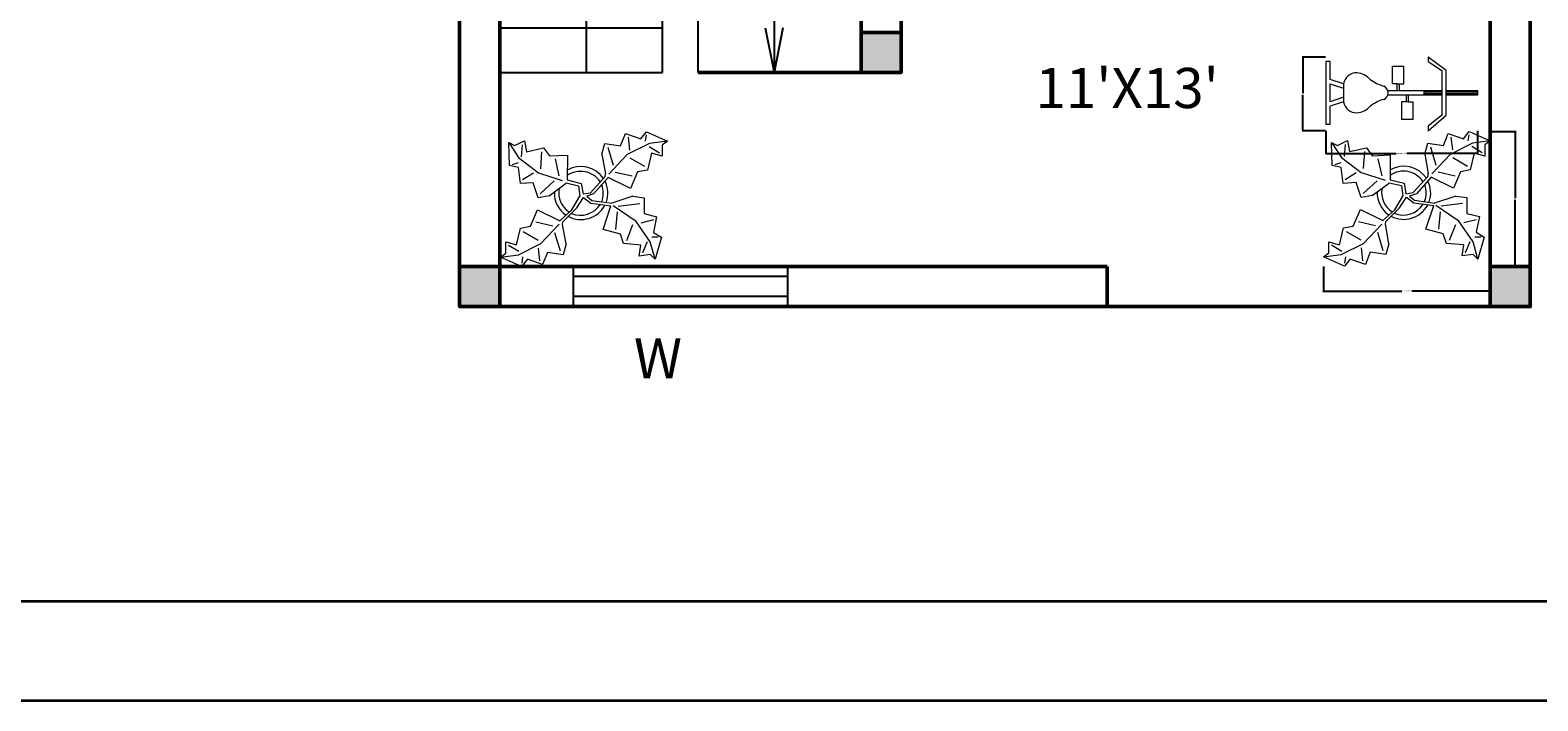
# Model space of a CAD drawing. Units: inches. Extents: x 28637 to 29820, y 17246 to 17928.
# Tile 3 of 6: x 28996 to 29334, y 17246 to 17397. Entities that reach past the tile are written whole.
import ezdxf

# ---------------------------------------------------------------- set-up
doc = ezdxf.new("R2010")
doc.units = ezdxf.units.IN
for name, color, linetype, lineweight in [('A-ANNO-DIMS', 2, 'Continuous', 18), ('A-ANNO-TEXT', 7, 'Continuous', 25), ('A-ANNO-TTLB', 7, 'Continuous', 35), ('A-AREA-IDEN', 30, 'Continuous', 25), ('A-COLS', 1, 'Continuous', 50), ('A-FLOR-STRS', 3, 'Continuous', 25), ('A-FURN', 8, 'Continuous', 18), ('A-GLAZ', 4, 'Continuous', 25), ('A-WALL', 7, 'Continuous', 50)]:
    doc.layers.add(name, color=color, linetype=linetype, lineweight=lineweight)
doc.styles.get("Standard").update_dxf_attribs({"font": 'arial.ttf'})
doc.dimstyles.get("Standard").update_dxf_attribs({"dimtxt": 0.18, "dimasz": 0.18, "dimexe": 0.18, "dimexo": 0.0625, "dimgap": 0.09, "dimtad": 0, "dimtih": 1, "dimtoh": 1, "dimdec": 4, "dimzin": 0, "dimdsep": 46, "dimtxsty": 'Standard', "dimcen": 0.09, "dimadec": 0, "dimazin": 0, "dimtfac": 1, "dimtdec": 4, "dimtofl": 0, "dimtmove": 0, "dimatfit": 3, "dimfxl": 1, "dimtolj": 1, "dimtzin": 0, "dimarcsym": 0})

# ---------------------------------------------------------------- blocks, each defined once
blk = doc.blocks.new('Exercise Bike')
for p, q in [((-0.75, 10), (-0.75, 17)), ((-0.75, 17), (0.25, 17)), ((-0.5, 17), (-0.5, 9.9929)), ((-0.25, 10), (-0.25, 17)), ((0, 17), (0, 9.9929)), ((0.25, 17), (0.25, 10)), ((-5.25, 10), (-8.25, 6)), ((-7.25, 6), (-5.25, 9)), ((-0.75, 10), (-5.25, 10)), ((-5.25, 9), (4.75, 9)), ((4.75, 10), (-0.75, 10)), ((-0.75, 5), (-0.75, 9)), ((-0.5, 8.9396), (-0.5, 5)), ((-0.25, 5), (-0.25, 9)), ((0, 8.9396), (0, 5)), ((0.25, 9), (0.25, 5)), ((8.25, 6), (4.75, 10)), ((4.75, 9), (7.25, 6)), ((-8.25, 6), (-7.25, 6)), ((-0.75, -3.0635), (-0.75, 5)), ((-0.75, 5), (0.25, 5)), ((0.25, 5), (0.25, -3.0635)), ((7.25, 6), (8.25, 6)), ((-6.25, -2), (-6.25, 0.5)), ((-2.25, 0.5), (-6.25, 0.5)), ((-2.25, -0.5), (-2.25, 0.5)), ((0.25, 1.5), (1.75, 1.5)), ((0.25, 1), (1.75, 1)), ((1.75, 2.5), (5.75, 2.5)), ((1.75, 1.5), (1.75, 2.5)), ((1.75, 1.5), (1.75, 0)), ((1.75, 0), (5.75, 0)), ((5.75, 2.5), (5.75, 0)), ((-2.25, -2), (-6.25, -2)), ((-2.25, -0.5), (-0.75, -0.5)), ((-2.25, -1), (-2.25, -0.5)), ((-2.25, -1), (-2.25, -2)), ((-0.75, -1), (-2.25, -1)), ((-2.25, -13), (-3.25, -16)), ((-2.25, -16), (-1.25, -13)), ((-2.25, -13), (1.75, -13)), ((0.75, -13), (1.75, -16)), ((1.75, -13), (2.75, -16)), ((-7.25, -16), (-7.25, -17)), ((-4.75, -16), (-7.25, -16)), ((-3.25, -16), (-4.75, -16)), ((1.75, -16), (-2.25, -16)), ((6.75, -16), (2.75, -16)), ((6.75, -17), (6.75, -16)), ((-7.25, -17), (6.75, -17))]:
    blk.add_line(p, q)
for centre, radius, start, end in [((-0.25, -4.625), 1.625, 22.61987, 157.3801), ((-9.6692, -1.9154), 8.1889, 321.6175, 345.2525), ((9.1691, -1.9154), 8.1889, 194.7476, 218.3825), ((0.1685, -10.5843), 4.9531, 133.6443, 173.2256), ((-1.7006, -10.0005), 3.0494, 179.9906, 259.6205), ((1.2006, -10.0005), 3.0494, 280.3795, 0.009389), ((-0.6686, -10.5843), 4.9531, 6.774486, 46.35562)]:
    blk.add_arc(centre, radius, start, end)
blk = doc.blocks.new('Plant - Rubber or Philodendron')
for p, q in [((13.3837, 12.301), (14.68, 13.9039)), ((14.68, 13.9039), (19.3848, 11.8146)), ((-16.2005, 11.4774), (-13.9899, 8.1064)), ((-16.2005, 11.4774), (-14.8639, 10.7964)), ((-16.0159, 6.3329), (-16.2005, 11.4774)), ((-14.8639, 10.7964), (-12.6195, 11.8975)), ((-13.3174, 8.325), (-13.0735, 11.0065)), ((-12.6195, 11.8975), (-12.1909, 9.4345)), ((-12.1909, 9.4345), (-8.3829, 10.3)), ((-8.3829, 10.3), (-7.0549, 8.501)), ((4.6914, 8.8812), (5.3859, 11.2828)), ((5.3859, 11.2828), (8.8871, 10.7908)), ((5.9878, 10.4842), (7.1971, 6.3869)), ((8.8871, 10.7908), (9.9809, 13.4933)), ((9.9809, 13.4933), (13.3837, 12.301)), ((15.3859, 11.3055), (10.3916, 8.7942)), ((10.5828, 12.6946), (10.8893, 9.7953)), ((14.5816, 13.2037), (14.3848, 11.8033)), ((15.2875, 10.6053), (17.5907, 9.2105)), ((19.3848, 11.8146), (15.3859, 11.3055)), ((19.3848, 11.8146), (18.1868, 10.9119)), ((18.1868, 10.9119), (18.1925, 8.4119)), ((-15.3434, 6.5514), (-13.9984, 6.9884)), ((-13.9899, 8.1064), (-9.5434, 4.7185)), ((-8.8369, 9.409), (-9.0894, 5.6095)), ((-7.0549, 8.501), (-3.0284, 8.6941)), ((-4.8529, 4.012), (-5.7184, 7.82)), ((-3.0284, 8.6941), (-3.0709, 3.1041)), ((4.6914, 8.8812), (5.5014, 4.4831)), ((10.3916, 8.7942), (6.2847, 4.4028)), ((14.2977, 6.1031), (10.9934, 7.9956)), ((15.7909, 9.1065), (14.8995, 5.3044)), ((18.1925, 8.4119), (15.7909, 9.1065)), ((-14.0069, 5.8704), (-16.0159, 6.3329)), ((-13.5868, 2.2894), (-14.0069, 5.8704)), ((-13.1329, 3.1804), (-10.6614, 4.727)), ((-9.5434, 4.7185), (-4.1917, 2.9888)), ((2.1141, 0.2298), (5.4346, 3.9146)), ((6.1032, 3.6844), (2.8262, -0.031)), ((5.4346, 3.9146), (5.5014, 4.4831)), ((11.1089, 1.1958), (6.1032, 3.6844)), ((7.7005, 4.8881), (11.5025, 3.9967)), ((12.7005, 4.8994), (11.1089, 1.1958)), ((14.8995, 5.3044), (12.7005, 4.8994)), ((-10.6784, 2.491), (-13.5868, 2.2894)), ((-9.5858, -0.8715), (-10.6784, 2.491)), ((-9.1318, 0.0195), (-5.9793, 2.9025)), ((-7.1228, -0.443), (-3.5248, 2.2131)), ((-3.5248, 2.2131), (-3.3011, 2.4355)), ((-3.3011, 2.4355), (-0.5306, 1.7947)), ((-3.0709, 3.1041), (0.0797, 2.3163)), ((-0.5306, 1.7947), (-0.2255, -0.5527)), ((-0.5306, 1.7947), (-0.5306, 1.7947)), ((0.0797, 2.3163), (0.4866, -0.031)), ((0.4866, -0.031), (2.1141, 0.2298)), ((-7.1228, -0.443), (-9.5858, -0.8715)), ((-4.0579, -6.2781), (-0.9375, -3.1608)), ((-2.019, -3.6148), (-0.2255, -0.5527)), ((-0.9375, -3.1608), (0.5883, -0.8135)), ((0.5883, -0.8135), (2.2447, -2.0916)), ((2.8262, -0.031), (1.3003, -0.5527)), ((1.3003, -0.5527), (2.4193, -1.4655)), ((2.2447, -2.0916), (6.7108, -2.6626)), ((2.4193, -1.4655), (6.895, -2.1175)), ((4.943, -7.9659), (6.7108, -2.6626)), ((11.6605, -0.5413), (6.895, -2.1175)), ((12.3677, -6.1981), (7.219, -2.6772)), ((8.3544, -2.7453), (13.1973, -2.1704)), ((11.6605, -0.5413), (14.1354, -0.8948)), ((14.1354, -0.8948), (14.1354, -4.4304)), ((-11.3237, -7.2629), (-9.7321, -3.5593)), ((-6.3237, -7.2516), (-10.1257, -6.3602)), ((-9.7321, -3.5593), (-4.7264, -6.0479)), ((-2.019, -3.6148), (-4.7264, -6.0479)), ((-4.1246, -6.8466), (-4.0579, -6.2781)), ((8.125, -4.0768), (7.7715, -7.9659)), ((15.5496, -10.7943), (12.3677, -6.1981)), ((16.2567, -5.8446), (13.4283, -6.5517)), ((14.1354, -4.4304), (16.9638, -5.1375)), ((16.9638, -5.1375), (16.2567, -8.673)), ((-14.4141, -11.4699), (-13.5228, -7.6679)), ((-13.5228, -7.6679), (-11.3237, -7.2629)), ((-12.921, -8.4665), (-9.6166, -10.359)), ((-9.0148, -11.1577), (-4.9047, -6.8122)), ((-4.611, -12.8477), (-5.8203, -8.7504)), ((-3.3146, -11.2447), (-4.1246, -6.8466)), ((8.8321, -9.0266), (4.943, -7.9659)), ((9.5392, -11.1479), (8.8321, -9.0266)), ((10.2463, -10.4408), (11.6605, -6.9053)), ((17.3174, -9.7337), (15.9032, -9.7337)), ((16.2567, -8.673), (18.0245, -9.7337)), ((18.0245, -9.7337), (16.6103, -14.6834)), ((-18.008, -14.1781), (-16.8101, -13.2754)), ((-16.8157, -10.7754), (-14.4141, -11.4699)), ((-16.8101, -13.2754), (-16.8157, -10.7754)), ((-13.9107, -12.9688), (-16.2139, -11.574)), ((-14.0091, -13.669), (-9.0148, -11.1577)), ((-9.206, -15.0581), (-9.5126, -12.1588)), ((-7.5103, -13.1543), (-8.6042, -15.8568)), ((-4.0092, -13.6463), (-7.5103, -13.1543)), ((-3.3146, -11.2447), (-4.0092, -13.6463)), ((13.4283, -11.5015), (9.5392, -11.1479)), ((13.0748, -13.9763), (13.4283, -11.5015)), ((14.8425, -10.7943), (13.7819, -13.2692)), ((16.6103, -14.6834), (15.5496, -10.7943)), ((-18.008, -14.1781), (-14.0091, -13.669)), ((-13.3032, -16.2674), (-18.008, -14.1781)), ((-12.0069, -14.6645), (-13.3032, -16.2674)), ((-13.2048, -15.5672), (-13.008, -14.1668)), ((-8.6042, -15.8568), (-12.0069, -14.6645)), ((15.5496, -13.6228), (13.0748, -13.9763)), ((16.6103, -14.6834), (15.5496, -13.6228))]:
    blk.add_line(p, q)
for centre, radius, start, end in [((0, 0), 6.1275, 34.37569, 120.1028), ((-0.0601, -0.2075), 5.2461, 33.82192, 124.9414), ((0.0308, 0.1664), 6, 178.6147, 235.1169), ((0.0308, 0.1664), 5, 168.1647, 238.6725), ((-0.2664, 0.1682), 5.2775, 338.4094, 20.03007), ((-0.098, 0.1364), 6.1288, 341.2017, 26.09184), ((-0.0234, 0.3825), 6.1492, 242.5812, 331.2714), ((-0.1102, 0.4886), 5.2883, 247.3711, 327.472)]:
    blk.add_arc(centre, radius, start, end)
blk = doc.blocks.new('STAIR')
for p, q in [((28799.14, 17387.25), (28799.14, 17499.75)), ((28807.14, 17387.25), (28807.14, 17499.75)), ((28762.64, 17467.25), (28799.14, 17467.25)), ((28782.14, 17387.25), (28782.14, 17467.25)), ((28824.14, 17467.25), (28824.14, 17387.25)), ((28762.64, 17457.25), (28799.14, 17457.25)), ((28762.64, 17447.25), (28799.14, 17447.25)), ((28762.64, 17437.25), (28799.14, 17437.25)), ((28762.64, 17427.25), (28799.14, 17427.25)), ((28762.64, 17417.25), (28799.14, 17417.25)), ((28762.64, 17407.25), (28799.14, 17407.25)), ((28762.64, 17397.25), (28799.14, 17397.25)), ((28822.14, 17397.25), (28824.14, 17387.25)), ((28826.14, 17397.25), (28824.14, 17387.25)), ((28762.64, 17387.25), (28799.14, 17387.25))]:
    blk.add_line(p, q)
blk.add_arc((28803.14, 17467.25), 21, 0, 180)
blk = doc.blocks.new('*D34')
at = {"layer": 'A-ANNO-DIMS', "color": 0, "lineweight": -2, "transparency": 16777216}
for p, q in [((29285.52, 17343.76), (29285.52, 17338.03)), ((29322.91, 17343.76), (29322.91, 17338.03)), ((29285.7, 17338.21), (29303.07, 17338.21)), ((29322.73, 17338.21), (29305.35, 17338.21))]:
    blk.add_line(p, q, dxfattribs=at)
at = {"layer": 'A-ANNO-DIMS', "color": 0, "transparency": 16777216}
for points in [[(29285.7, 17338.24), (29285.7, 17338.18), (29285.52, 17338.21)], [(29322.73, 17338.24), (29322.73, 17338.18), (29322.91, 17338.21)]]:
    blk.add_solid(points, dxfattribs=at)
at = {"layer": 'Defpoints', "color": 0, "transparency": 16777216}
for p in [(29285.52, 17343.82), (29322.91, 17343.82), (29322.91, 17338.21)]:
    blk.add_point(p, dxfattribs=at)
at = {"layer": 'A-ANNO-DIMS', "color": 0, "transparency": 16777216, "insert": (29304.21, 17338.21), "char_height": 0.18, "attachment_point": 5}
blk.add_mtext('\\A1;PLANTER 37 TYP.', dxfattribs=at)
blk = doc.blocks.new('*D35')
at = {"layer": 'A-ANNO-DIMS', "color": 0, "lineweight": -2, "transparency": 16777216}
for p, q in [((29322.97, 17373.99), (29328.7, 17373.99)), ((29328.52, 17373.81), (29328.52, 17359.09)), ((29328.52, 17344), (29328.52, 17358.72)), ((29322.97, 17343.82), (29328.7, 17343.82))]:
    blk.add_line(p, q, dxfattribs=at)
at = {"layer": 'A-ANNO-DIMS', "color": 0, "transparency": 16777216}
for points in [[(29328.49, 17373.81), (29328.55, 17373.81), (29328.52, 17373.99)], [(29328.49, 17344), (29328.55, 17344), (29328.52, 17343.82)]]:
    blk.add_solid(points, dxfattribs=at)
at = {"layer": 'Defpoints', "color": 0, "transparency": 16777216}
for p in [(29322.91, 17373.99), (29328.52, 17373.99), (29322.91, 17343.82)]:
    blk.add_point(p, dxfattribs=at)
at = {"layer": 'A-ANNO-DIMS', "color": 0, "transparency": 16777216, "insert": (29328.52, 17358.9), "char_height": 0.18, "attachment_point": 5}
blk.add_mtext('\\A1;30 TYP.', dxfattribs=at)
blk = doc.blocks.new('*D60')
at = {"layer": 'A-ANNO-DIMS', "color": 0, "lineweight": -2, "transparency": 16777216}
for p, q in [((29286.02, 17374.14), (29286.02, 17368.92)), ((29320.02, 17374.14), (29320.02, 17368.92)), ((29286.2, 17369.1), (29301.82, 17369.1)), ((29319.84, 17369.1), (29304.23, 17369.1))]:
    blk.add_line(p, q, dxfattribs=at)
at = {"layer": 'A-ANNO-DIMS', "color": 0, "transparency": 16777216}
for points in [[(29286.2, 17369.13), (29286.2, 17369.07), (29286.02, 17369.1)], [(29319.84, 17369.13), (29319.84, 17369.07), (29320.02, 17369.1)]]:
    blk.add_solid(points, dxfattribs=at)
at = {"layer": 'Defpoints', "color": 0, "transparency": 16777216}
for p in [(29286.02, 17374.2), (29320.02, 17374.2), (29320.02, 17369.1)]:
    blk.add_point(p, dxfattribs=at)
at = {"layer": 'A-ANNO-DIMS', "color": 0, "transparency": 16777216, "insert": (29303.02, 17369.1), "char_height": 0.18, "attachment_point": 5}
blk.add_mtext('\\A1;EXERCISE BIKE 34', dxfattribs=at)
blk = doc.blocks.new('*D61')
at = {"layer": 'A-ANNO-DIMS', "color": 0, "lineweight": -2, "transparency": 16777216}
for p, q in [((29285.96, 17390.7), (29280.74, 17390.7)), ((29280.92, 17390.52), (29280.92, 17382.63)), ((29280.92, 17374.38), (29280.92, 17382.27)), ((29285.96, 17374.2), (29280.74, 17374.2))]:
    blk.add_line(p, q, dxfattribs=at)
at = {"layer": 'A-ANNO-DIMS', "color": 0, "transparency": 16777216}
for points in [[(29280.89, 17390.52), (29280.95, 17390.52), (29280.92, 17390.7)], [(29280.89, 17374.38), (29280.95, 17374.38), (29280.92, 17374.2)]]:
    blk.add_solid(points, dxfattribs=at)
at = {"layer": 'Defpoints', "color": 0, "transparency": 16777216}
for p in [(29286.02, 17390.7), (29280.92, 17374.2), (29286.02, 17374.2)]:
    blk.add_point(p, dxfattribs=at)
at = {"layer": 'A-ANNO-DIMS', "color": 0, "transparency": 16777216, "insert": (29280.92, 17382.45), "char_height": 0.18, "attachment_point": 5}
blk.add_mtext('\\A1;17', dxfattribs=at)

msp = doc.modelspace()

# ---------------------------------------------------------------- hatches: boundary and pattern name
at = {"layer": 'A-COLS'}
h = msp.add_hatch(color=256, dxfattribs=at)
h.dxf.hatch_style = 1
h.paths.add_polyline_path([(29181.87, 17396.25), (29181.87, 17387.25), (29190.87, 17387.25), (29190.87, 17396.25)])
h = msp.add_hatch(color=256, dxfattribs=at)
h.dxf.hatch_style = 1
h.paths.add_polyline_path([(29091.87, 17343.75), (29091.87, 17334.75), (29100.87, 17334.75), (29100.87, 17343.75)])
h = msp.add_hatch(color=256, dxfattribs=at)
h.dxf.hatch_style = 1
h.paths.add_polyline_path([(29322.87, 17343.75), (29322.87, 17334.75), (29331.87, 17334.75), (29331.87, 17343.75)])

# ---------------------------------------------------------------- linework, layer by layer
at = {"layer": 'A-ANNO-TTLB'}
for points in [[(28637.03, 17927.97), (29820.02, 17927.97), (29820.02, 17246.37), (28637.03, 17246.37)], [(28663.78, 17907.18), (29794.75, 17907.18), (29794.75, 17268.65), (28663.78, 17268.65)]]:
    msp.add_lwpolyline(points, close=True, dxfattribs=at)
at = {"layer": 'A-COLS'}
for points in [[(29181.87, 17396.25), (29190.87, 17396.25), (29190.87, 17387.25), (29181.87, 17387.25)], [(29091.87, 17343.75), (29100.87, 17343.75), (29100.87, 17334.75), (29091.87, 17334.75)], [(29322.87, 17343.75), (29331.87, 17343.75), (29331.87, 17334.75), (29322.87, 17334.75)]]:
    msp.add_lwpolyline(points, close=True, dxfattribs=at)
at = {"layer": 'A-GLAZ'}
for p, q in [((29117.37, 17343.75), (29117.37, 17334.75)), ((29165.37, 17343.75), (29165.37, 17334.75)), ((29165.37, 17341.5), (29117.37, 17341.5)), ((29165.37, 17337), (29117.37, 17337))]:
    msp.add_line(p, q, dxfattribs=at)
at = {"layer": 'A-WALL'}
for p, q in [((29091.87, 17334.75), (29091.87, 17814.75)), ((29331.87, 17814.75), (29331.87, 17334.75)), ((29100.87, 17343.75), (29100.87, 17499.75)), ((29181.87, 17499.75), (29181.87, 17387.25)), ((29190.87, 17485.35), (29190.87, 17387.25)), ((29322.87, 17475.75), (29322.87, 17343.75)), ((29145.37, 17387.25), (29190.87, 17387.25)), ((29237.05, 17343.75), (29100.87, 17343.75)), ((29181.87, 17343.75), (29100.87, 17343.75)), ((29237.05, 17343.75), (29237.05, 17334.75)), ((29331.87, 17334.75), (29091.87, 17334.75)), ((29331.87, 17334.75), (29322.87, 17334.75))]:
    msp.add_line(p, q, dxfattribs=at)

# ---------------------------------------------------------------- block references
at = {"layer": 'A-FLOR-STRS'}
msp.add_blockref('STAIR', (338.22, 0), dxfattribs=at)
at = {"layer": 'A-FURN', "rotation": 270}
msp.add_blockref('Exercise Bike', (29303.02, 17382.45), dxfattribs=at)
at = {"layer": 'A-FURN'}
for p in [(29119.09, 17360.05), (29303.52, 17360.09)]:
    msp.add_blockref('Plant - Rubber or Philodendron', p, dxfattribs=at)

# ---------------------------------------------------------------- texts
at = {"layer": 'A-ANNO-TEXT'}
msp.add_text('    W', height=9, dxfattribs=at).set_placement((29119.96, 17318.65))
at = {"layer": 'A-AREA-IDEN'}
msp.add_text("       11'X13'", height=9, dxfattribs=at).set_placement((29201.7, 17379.28))

# ---------------------------------------------------------------- dimensions: what is measured, and where the dimension line sits
at = {"layer": 'A-ANNO-DIMS'}
dim = msp.add_linear_dim(base=(29280.92159739, 17374.20140273), p1=(29286.02159739, 17390.70140273), p2=(29286.02159739, 17374.20140273), angle=270, dimstyle='Standard', override={"dimdec": 0, "dimlfac": 1, "dimrnd": 0, "dimzin": 0, "dimdsep": 46, "dimlunit": 2}, dxfattribs=at)
dim.commit()
dim.dimension.update_dxf_attribs({"geometry": '*D61', "text_midpoint": (29280.92159739, 17382.45140273)})
for base, p1, p2, text, picture, middle in [((29320.02, 17369.1), (29286.02, 17374.2), (29320.02, 17374.2), 'EXERCISE BIKE <>', '*D60', (29303.02, 17369.1)), ((29322.91, 17338.21), (29285.52, 17343.82), (29322.91, 17343.82), 'PLANTER <> TYP.', '*D34', (29304.21, 17338.21))]:
    dim = msp.add_linear_dim(base=base, p1=p1, p2=p2, text=text, dimstyle='Standard', override={"dimdec": 0, "dimlfac": 1, "dimrnd": 0, "dimzin": 0, "dimdsep": 46, "dimlunit": 2}, dxfattribs=at)
    dim.commit()
    dim.dimension.update_dxf_attribs({"geometry": picture, "text_midpoint": middle})
dim = msp.add_linear_dim(base=(29328.52, 17373.99), p1=(29322.91, 17343.82), p2=(29322.91, 17373.99), angle=90, text='<> TYP.', dimstyle='Standard', override={"dimdec": 0, "dimlfac": 1, "dimrnd": 0, "dimzin": 0, "dimdsep": 46, "dimlunit": 2}, dxfattribs=at)
dim.commit()
dim.dimension.update_dxf_attribs({"geometry": '*D35', "text_midpoint": (29328.52, 17358.9)})

doc.saveas('drawing.dxf')
